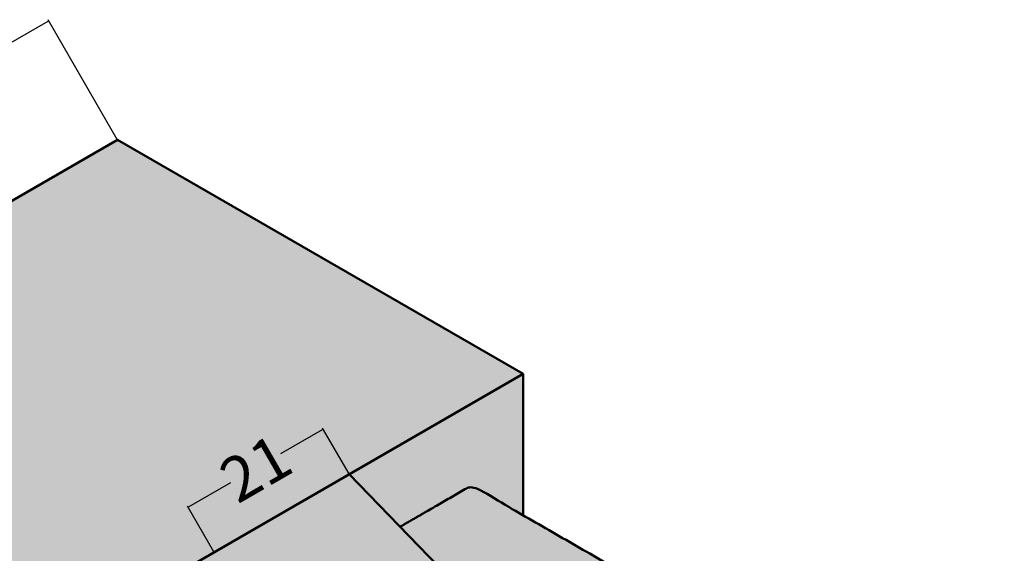
# Model space of a CAD drawing. Units: millimetres. Extents: x -24 to 183, y 0 to 191.
# Tile 1 of 1: x 51 to 183.4, y 119.6 to 191.4. Entities that reach past the tile are written whole.
import ezdxf

# ---------------------------------------------------------------- set-up
doc = ezdxf.new("R2010")
doc.units = ezdxf.units.MM
doc.header["$MEASUREMENT"] = 0
for name, color, linetype, lineweight in [('M-DIMS', 2, 'Continuous', 25), ('M-HATC', 7, 'Continuous', 18), ('M-OUTL', 7, 'Continuous', 50)]:
    doc.layers.add(name, color=color, linetype=linetype, lineweight=lineweight)
doc.styles.get("Standard").update_dxf_attribs({"font": 'arial.ttf'})
doc.dimstyles.get("Standard").update_dxf_attribs({"dimtxt": 6, "dimasz": 0.18, "dimexe": 0.18, "dimexo": 0.0625, "dimgap": 0.09, "dimtad": 0, "dimtoh": 1, "dimdec": 0, "dimzin": 0, "dimdsep": 46, "dimtxsty": 'Standard', "dimcen": 0.09, "dimadec": 0, "dimazin": 0, "dimtfac": 1, "dimtdec": 0, "dimtofl": 0, "dimtmove": 0, "dimatfit": 3, "dimfxl": 1, "dimtolj": 1, "dimtzin": 0, "dimarcsym": 0})

# ---------------------------------------------------------------- blocks, each defined once
blk = doc.blocks.new('*D1')
at = {"layer": 'Defpoints', "color": 0, "transparency": 16777216}
for p in [(91.82160620577477, 136.269941405224), (95.31936918098474, 130.2116382193271), (77.13283570151162, 119.7116382193271)]:
    blk.add_point(p, dxfattribs=at)
at = {"layer": 'M-DIMS', "color": 0, "lineweight": -2, "transparency": 16777216}
for p, q in [((91.66572163309357, 136.179941405224), (86.07071311753079, 132.9496617326455)), ((95.28811918098474, 130.2657648070636), (91.73160620577475, 136.4258259779052)), ((73.79095729898287, 125.859941405224), (79.38596581454564, 129.0902210778024)), ((77.10158570151162, 119.7657648070636), (73.54507272630167, 125.9258259779052))]:
    blk.add_line(p, q, dxfattribs=at)
at = {"layer": 'M-DIMS', "color": 0, "transparency": 16777216}
for points in [[(91.6507216330936, 136.2059221673375), (91.68072163309358, 136.1539606431104), (91.82160620577477, 136.269941405224)], [(73.77595729898287, 125.8859221673375), (73.80595729898288, 125.8339606431105), (73.63507272630167, 125.769941405224)]]:
    blk.add_solid(points, dxfattribs=at)
at = {"layer": 'M-DIMS', "color": 0, "transparency": 16777216, "insert": (82.72833946603824, 131.019941405224), "char_height": 6, "attachment_point": 5, "rotation": 30.00000000000005}
blk.add_mtext('\\A1;21', dxfattribs=at)
blk = doc.blocks.new('*D3')
at = {"layer": 'Defpoints', "color": 0, "transparency": 16777216}
for p in [(54.90112838051421, 191.2180848382955), (64.142454644745, 175.211638219327), (-0.8094506390879203, 137.7116382193271)]:
    blk.add_point(p, dxfattribs=at)
at = {"layer": 'M-DIMS', "color": 0, "lineweight": -2, "transparency": 16777216}
for p, q in [((54.745243807833, 191.1280848382955), (26.22301022659634, 174.6607656022791)), ((64.111204644745, 175.2657648070636), (54.8111283805142, 191.3739694109767)), ((-9.89489233063751, 153.8080848382955), (18.62734125059916, 170.2754040743118)), ((-0.8407006390879203, 137.7657648070636), (-10.14077690331872, 153.8739694109767))]:
    blk.add_line(p, q, dxfattribs=at)
at = {"layer": 'M-DIMS', "color": 0, "transparency": 16777216}
for points in [[(54.730243807833, 191.154065600409), (54.760243807833, 191.102104076182), (54.90112838051421, 191.2180848382955)], [(-9.909892330637511, 153.834065600409), (-9.87989233063751, 153.7821040761819), (-10.05077690331871, 153.7180848382955)]]:
    blk.add_solid(points, dxfattribs=at)
at = {"layer": 'M-DIMS', "color": 0, "transparency": 16777216, "insert": (22.42517573859776, 172.4680848382955), "char_height": 6, "attachment_point": 5, "rotation": 29.999999999999993}
blk.add_mtext('\\A1;75', dxfattribs=at)

msp = doc.modelspace()

# ---------------------------------------------------------------- hatches: boundary and pattern name
at = {"layer": 'M-HATC'}
h = msp.add_hatch(color=256, dxfattribs=at)
h.set_gradient(color1=(244, 238, 81), color2=(244, 238, 81), tint=1)
h.paths.add_polyline_path([(64.14245464474502, 175.211638219327), (-0.8094506390879131, 137.7116382193271), (53.75014979933173, 106.2116382193271), (118.7020550831646, 143.7116382193271)])
edge = h.paths.add_edge_path()
edge.add_line((95.31936918098478, 130.2116382193271), (77.13283570151161, 119.7116382193271))
edge.add_spline(control_points=[(77.13283570151158, 119.7116382193271), (89.17924906810929, 107.2566382193724), (101.2256624347508, 94.80163821937239)], knot_values=[5.356194490192345, 5.356194490192345, 5.356194490192345, 6.356194490188707, 6.356194490192345, 6.356194490192345], weights=[1, 1, 1], degree=2, periodic=0)
edge.add_spline(control_points=[(101.2256624347947, 94.80163821932707), (110.3189291745312, 100.051638219327), (119.4121959142679, 105.301638219327)], knot_values=[6.356194490188707, 6.356194490192345, 6.356194490192345, 7.356194490192345, 7.356194490192345, 7.356194490192345], weights=[1, 1, 1], degree=2, periodic=0)
edge.add_line((119.4121959142679, 105.3016382193271), (95.31936918098478, 130.2116382193271))
edge = h.paths.add_edge_path()
edge.add_spline(control_points=[(150.7449950231889, 106.2116382193271), (134.7235250531767, 115.4616382193271), (118.7020550831646, 124.7116382193271)], knot_values=[3.356194490192345, 3.356194490192345, 3.356194490192345, 4.178416712414569, 4.178416712414569, 4.178416712414569], weights=[1, 1, 1], degree=2, periodic=0)
edge.add_spline(control_points=[(118.7020550831646, 124.7116382193271), (115.2379534680269, 126.7116382193271), (111.7738518528891, 128.7116382193271)], knot_values=[4.178416712414569, 4.178416712414569, 4.178416712414569, 4.356194490192345, 4.356194490192345, 4.356194490192345], weights=[1, 1, 1], degree=2, periodic=0)
edge.add_spline(control_points=[(111.7738518528891, 128.7116382193271), (106.960071285434, 125.9324007128871), (102.1462907179789, 123.1531632064471)], knot_values=[4.356194490192345, 4.356194490192345, 4.356194490192345, 5.356194490192345, 5.356194490192345, 5.356194490192345], weights=[1, 1, 1], degree=2, periodic=0)
edge.add_line((102.1462907179789, 123.1531632064471), (119.4121959142679, 105.301638219327))
edge.add_spline(control_points=[(119.4121959142679, 105.301638219327), (126.8513541327762, 101.006638219327), (134.2905123512845, 96.71163821932709)], knot_values=[7.356194490192345, 7.356194490192345, 7.356194490192345, 8.356194490192346, 8.356194490192346, 8.356194490192346], weights=[1, 1, 1], degree=2, periodic=0)
edge.add_spline(control_points=[(134.2905123512845, 96.71163821932709), (158.0953395036126, 82.96791485491796), (161.6862132372617, 53.72180942535438), (165.2770869709107, 24.47570399579081), (142.5556009483879, 29.39608484008592)], knot_values=[8.356194490192346, 8.356194490192346, 8.356194490192346, 9.775566349411587, 9.775566349411587, 11.19493820863083, 11.19493820863083, 11.19493820863083], weights=[1, 0.7585665602715825, 1, 0.7585665602715825, 1], degree=2, periodic=0)
edge.add_spline(control_points=[(153.8864302935499, 30.77051272237281), (162.1136716295021, 35.52051272237281), (170.3409129654543, 40.2705127223728)], knot_values=[0, 0, 0, 1, 1, 1], weights=[1, 1, 1], degree=2, periodic=0)
edge.add_spline(control_points=[(170.3409129654543, 40.2705127223728), (183.4344867248955, 47.83009105704043), (176.3482956693094, 71.67543553482938), (169.2621046137232, 95.5207800126183), (150.7449950231889, 106.2116382193271)], knot_values=[1, 1, 1, 2.178097245096171, 2.178097245096171, 3.356194490192345, 3.356194490192345, 3.356194490192345], weights=[1, 0.831469612302545, 1, 0.831469612302545, 1], degree=2, periodic=0)
edge = h.paths.add_edge_path(flags=17)
edge.add_spline(control_points=[(134.2905123512845, 96.71163821932709), (126.8513541327762, 101.006638219327), (119.4121959142679, 105.301638219327)], knot_values=[7.356194490192345, 7.356194490192345, 7.356194490192345, 8.356194490192346, 8.356194490192346, 8.356194490192346], weights=[1, 1, 1], degree=2, periodic=0)
edge.add_line((119.4121959142679, 105.301638219327), (119.4121959142679, 84.07281383496964))
edge.add_spline(control_points=[(119.4121959142679, 84.07281383496964), (123.0724490086632, 81.4513939238958), (126.4903518736498, 77.88262675949477)], knot_values=[2.966768687208849, 2.966768687208849, 2.966768687208849, 3.231438789490306, 3.231438789490306, 3.231438789490306], weights=[0.9680864183363699, 0.938243390584542, 0.9254123758008628], degree=2, periodic=0)
edge.add_ellipse((134.2905123512845, 64.71163821932709), major_axis=(7.654655446197426, -13.25825214724777), ratio=0.5773502691896262, start_angle=359.3650130620468, end_angle=540.634986937953, ccw=False)
edge.add_spline(control_points=[(141.7968427812057, 51.37100682201758), (145.5119247027769, 38.61436904653682), (142.5556009483879, 29.39608484008592)], knot_values=[1.485548755374229, 1.485548755374229, 1.485548755374229, 2.169061485720957, 2.169061485720957, 2.169061485720957], weights=[0.9974346422091759, 0.9011559533067647, 0.9183363162707197], degree=2, periodic=0)
edge.add_spline(control_points=[(142.5556009483879, 29.39608484008592), (165.2770869709107, 24.47570399579081), (161.6862132372617, 53.72180942535438), (158.0953395036126, 82.96791485491796), (134.2905123512845, 96.71163821932709)], knot_values=[8.356194490192342, 8.356194490192342, 8.356194490192342, 9.775566349411587, 9.775566349411587, 11.19493820863083, 11.19493820863083, 11.19493820863083], weights=[1, 0.7585665602715825, 1, 0.7585665602715825, 1], degree=2, periodic=0)
edge = h.paths.add_edge_path()
edge.add_spline(control_points=[(119.4121959142679, 105.301638219327), (110.3189291745312, 100.051638219327), (101.2256624347947, 94.80163821932707)], knot_values=[6.356194490188707, 6.356194490188707, 6.356194490188707, 7.356194490188707, 7.356194490188707, 7.356194490192345], weights=[1, 1, 1], degree=2, periodic=0)
edge.add_spline(control_points=[(101.2256624347947, 94.80163821932709), (108.664820653303, 90.5066382193271), (116.1039788718113, 86.21163821932711)], knot_values=[3.356194490192346, 3.356194490192346, 3.356194490192346, 3.737972267970123, 3.737972267970123, 3.737972267970123], weights=[1, 1, 1], degree=2, periodic=0)
edge.add_spline(control_points=[(116.1039788718113, 86.21163821932711), (117.7640226821475, 85.25321147856292), (119.4121959142679, 84.07281383496964)], knot_values=[3.231438789490306, 3.231438789490306, 3.231438789490306, 3.356194490192346, 3.356194490192346, 3.356194490192346], weights=[1, 0.9821533182474542, 0.9680864183363699], degree=2, periodic=0)
edge.add_line((119.4121959142679, 84.07281383496965), (119.4121959142679, 105.301638219327))
h.paths.add_polyline_path([(-0.8094506390879131, 137.7116382193271), (-0.8094506390879131, 117.7116382193271), (32.09951470472076, 98.71163821932709), (32.09951470472076, 63.71163821932707), (-0.8094506390879131, 82.71163821932709), (-0.8094506390879062, 62.71163821932709), (53.75014979933173, 31.21163821932709), (53.75014979933173, 106.2116382193271)])
h.paths.add_polyline_path([(32.09951470472076, 98.71163821932709), (29.50143849336745, 100.2116382193271), (-0.8094506390879203, 82.71163821932709), (32.09951470472076, 63.71163821932708)])
edge = h.paths.add_edge_path()
edge.add_spline(control_points=[(99.64949619990696, 57.21163821932711), (99.64949619990696, 66.96163821932711), (99.64949619990696, 76.71163821932711)], knot_values=[5.141592653589794, 5.141592653589794, 5.141592653589794, 5.446280153589794, 5.446280153589794, 5.446280153589794], weights=[1, 1, 1], degree=2, periodic=0)
edge.add_line((99.64949619990699, 76.7116382193271), (60.67835302960723, 99.2116382193271))
edge.add_spline(control_points=[(60.67835302960723, 99.2116382193271), (60.67835302960723, 67.2116382193271), (60.67835302960723, 35.2116382193271)], knot_values=[0, 0, 0, 1, 1, 1], weights=[1, 1, 1], degree=2, periodic=0)
edge.add_spline(control_points=[(60.67835302960723, 35.2116382193271), (80.16392461475712, 23.9616382193271), (99.64949619990699, 12.71163821932711)], knot_values=[1, 1, 1, 2, 2, 2], weights=[1, 1, 1], degree=2, periodic=0)
edge.add_spline(control_points=[(99.64949619990699, 12.7116382193271), (99.64949619990699, 22.4616382193271), (99.64949619990699, 32.2116382193271)], knot_values=[5.836905153589794, 5.836905153589794, 5.836905153589794, 6.141592653589794, 6.141592653589794, 6.141592653589794], weights=[1, 1, 1], degree=2, periodic=0)
edge.add_ellipse((99.64949619990699, 44.7116382193271), major_axis=(7.654655446197426, -13.25825214724777), ratio=0.5773502691896261, start_angle=150, end_angle=330, ccw=False)
edge = h.paths.add_edge_path(flags=17)
edge.add_spline(control_points=[(77.13283570151158, 119.7116382193271), (77.13283570151158, 114.2116382193271), (77.13283570151158, 108.711638219327)], knot_values=[4.356194490192345, 4.356194490192345, 4.356194490192345, 5.356194490192345, 5.356194490192345, 5.356194490192345], weights=[1, 1, 1], degree=2, periodic=0)
edge.add_spline(control_points=[(77.13283570151158, 108.711638219327), (89.17924906815313, 101.7566382193271), (101.2256624347947, 94.80163821932709)], knot_values=[3.737972267970123, 3.737972267970123, 3.737972267970123, 4.356194490192345, 4.356194490192345, 4.356194490192345], weights=[1, 1, 1], degree=2, periodic=0)
edge.add_spline(control_points=[(101.2256624347508, 94.80163821937239), (89.17924906810929, 107.2566382193724), (77.13283570151158, 119.7116382193271)], knot_values=[5.356194490192345, 5.356194490192345, 5.356194490195983, 6.356194490192345, 6.356194490192345, 6.356194490192345], weights=[1, 1, 1], degree=2, periodic=0)
edge = h.paths.add_edge_path()
edge.add_spline(control_points=[(119.2454141421726, 10.77051272237291), (121.8252656817894, 12.25999070323999), (123.649496199907, 14.85523175877608), (131.649496199907, 26.23642960525908), (123.649496199907, 46.8552317587761), (115.649496199907, 67.4740339122931), (99.64949619990696, 76.71163821932711)], knot_values=[2.780860556892677, 2.780860556892677, 2.780860556892677, 3.047197551196599, 3.047197551196599, 4.094395102393195, 4.094395102393195, 5.141592653589794, 5.141592653589794, 5.141592653589794], weights=[0.9491840326991366, 0.9659258262890693, 1, 0.8660254037844385, 1, 0.8660254037844385, 1], degree=2, periodic=0)
edge.add_spline(control_points=[(99.64949619990696, 76.71163821932711), (99.64949619990696, 66.96163821932711), (99.64949619990696, 57.21163821932711)], knot_values=[5.141592653589794, 5.141592653589794, 5.141592653589794, 5.446280153589794, 5.446280153589794, 5.446280153589794], weights=[1, 1, 1], degree=2, periodic=0)
edge.add_ellipse((99.64949619990699, 44.7116382193271), major_axis=(7.654655446197426, -13.25825214724777), ratio=0.5773502691896261, start_angle=330, end_angle=509.9999999999999, ccw=False)
edge.add_spline(control_points=[(99.64949619990699, 32.2116382193271), (99.64949619990699, 22.4616382193271), (99.64949619990699, 12.7116382193271)], knot_values=[5.836905153589794, 5.836905153589794, 5.836905153589794, 6.141592653589794, 6.141592653589794, 6.141592653589794], weights=[1, 1, 1], degree=2, periodic=0)
edge.add_spline(control_points=[(99.64949619990699, 12.71163821932711), (111.1285191633359, 6.084221221357497), (119.2454141421726, 10.77051272237291)], knot_values=[2, 2, 2, 2.780860556892677, 2.780860556892677, 2.780860556892677], weights=[1, 0.9000995774953693, 0.9491840326991366], degree=2, periodic=0)
edge = h.paths.add_edge_path()
edge.add_line((118.7020550831646, 143.7116382193271), (95.31936918098478, 130.2116382193271))
edge.add_line((95.31936918098478, 130.2116382193271), (102.1462907179789, 123.1531632064471))
edge.add_spline(control_points=[(102.1462907179789, 123.1531632064471), (106.960071285434, 125.9324007128871), (111.7738518528891, 128.7116382193271)], knot_values=[4.356194490192345, 4.356194490192345, 4.356194490192345, 5.356194490192345, 5.356194490192345, 5.356194490192345], weights=[1, 1, 1], degree=2, periodic=0)
edge.add_spline(control_points=[(111.7738518528891, 128.7116382193271), (115.2379534680269, 126.7116382193271), (118.7020550831646, 124.7116382193271)], knot_values=[4.178416712414568, 4.178416712414568, 4.178416712414568, 4.356194490192344, 4.356194490192344, 4.356194490192344], weights=[1, 1, 1], degree=2, periodic=0)
edge.add_line((118.7020550831646, 124.7116382193271), (118.7020550831646, 143.7116382193271))
h = msp.add_hatch(color=256, dxfattribs=at)
h.set_gradient(color1=(244, 238, 81), color2=(244, 238, 81), tint=1)
edge = h.paths.add_edge_path()
edge.add_spline(control_points=[(77.13283570151158, 108.711638219327), (77.13283570151158, 114.2116382193271), (77.13283570151158, 119.7116382193271)], knot_values=[4.356194490192345, 4.356194490192345, 4.356194490192345, 5.356194490192345, 5.356194490192345, 5.356194490192345], weights=[1, 1, 1], degree=2, periodic=0)
edge.add_line((77.13283570151158, 119.7116382193271), (53.75014979933173, 106.2116382193271))
edge.add_line((53.75014979933173, 106.2116382193271), (53.75014979933173, 31.21163821932707))
edge.add_line((53.75014979933173, 31.21163821932707), (60.67835302960723, 35.21163821932709))
edge.add_spline(control_points=[(60.67835302960723, 35.2116382193271), (60.67835302960723, 67.2116382193271), (60.67835302960723, 99.2116382193271)], knot_values=[0, 0, 0, 1, 1, 1], weights=[1, 1, 1], degree=2, periodic=0)
edge.add_line((60.67835302960723, 99.2116382193271), (77.13283570151158, 108.7116382193271))
edge = h.paths.add_edge_path()
edge.add_spline(control_points=[(129.6626567046299, 74.29200746748931), (128.2121653973336, 76.06903189246286), (126.674769139423, 77.68917768712181)], knot_values=[2.842732393323176, 2.842732393323176, 2.842732393323176, 2.959718296587445, 2.959718296587445, 2.959718296587445], weights=[0.9171223116143046, 0.9192697655211874, 0.9247408519506481], degree=2, periodic=0)
edge.add_spline(control_points=[(126.674769139423, 77.68917768712181), (126.5826958679184, 77.78620675354577), (126.4903518736499, 77.88262675949478)], knot_values=[2.959718296587445, 2.959718296587445, 2.959718296587445, 2.966768687208849, 2.966768687208849, 2.966768687208849], weights=[0.9247408519506481, 0.925070577972116, 0.9254123758008624], degree=2, periodic=0)
edge.add_spline(control_points=[(126.4903518736499, 77.88262675949478), (125.1497541063207, 79.2823977540787), (123.7600353652503, 80.54602783327896)], knot_values=[2.966768687208849, 2.966768687208849, 2.966768687208849, 3.069712263544142, 3.069712263544142, 3.069712263544142], weights=[0.9254123758008624, 0.9304030057906388, 0.9379672558727182], degree=2, periodic=0)
edge.add_spline(control_points=[(123.7600353652503, 80.54602783327896), (122.2074968153256, 81.95770514094174), (120.6136211690738, 83.18146756875178)], knot_values=[3.069712263544142, 3.069712263544142, 3.069712263544142, 3.18671441540082, 3.18671441540082, 3.18671441540082], weights=[0.9379672558727182, 0.946564524087908, 0.9584863481523173], degree=2, periodic=0)
edge.add_spline(control_points=[(120.6136211690738, 83.18146756875178), (120.0147834077447, 83.6412494559974), (119.4121959142679, 84.07281383496966)], knot_values=[3.18671441540082, 3.18671441540082, 3.18671441540082, 3.231438789490306, 3.231438789490306, 3.231438789490306], weights=[0.9584863481523173, 0.9630434961263034, 0.9680864183363697], degree=2, periodic=0)
edge.add_spline(control_points=[(119.4121959142679, 84.07281383496966), (119.0199233503353, 84.35375372714144), (118.6264656481512, 84.62244284625048)], knot_values=[3.231438789490306, 3.231438789490306, 3.231438789490306, 3.260806039297188, 3.260806039297188, 3.260806039297188], weights=[0.9680864183363697, 0.9713977392729884, 0.9749185064116943], degree=2, periodic=0)
edge.add_spline(control_points=[(118.6264656481512, 84.62244284625048), (117.3678455130209, 85.48194447380494), (116.1039788718113, 86.21163821932711)], knot_values=[3.260806039297188, 3.260806039297188, 3.260806039297188, 3.356194490192345, 3.356194490192345, 3.356194490192345], weights=[0.9749185064116943, 0.9863543924933733, 1], degree=2, periodic=0)
edge.add_spline(control_points=[(116.1039788718113, 86.21163821932711), (111.8084928690405, 88.6916382193271), (107.5130068662697, 91.1716382193271)], knot_values=[3.356194490192345, 3.356194490192345, 3.356194490192345, 3.57663893463679, 3.57663893463679, 3.57663893463679], weights=[1, 1, 1], degree=2, periodic=0)
edge.add_spline(control_points=[(107.5130068662697, 91.1716382193271), (104.3693346505321, 92.98663821932709), (101.2256624347947, 94.80163821932709)], knot_values=[3.57663893463679, 3.57663893463679, 3.57663893463679, 3.737972267970123, 3.737972267970123, 3.737972267970123], weights=[1, 1, 1], degree=2, periodic=0)
edge.add_spline(control_points=[(101.2256624347947, 94.80163821932709), (89.18162767796578, 101.7552649283114), (77.13759292113684, 108.7088916372958)], knot_values=[3.737972267970123, 3.737972267970123, 3.737972267970123, 4.356072419879845, 4.356072419879845, 4.356072419879845], weights=[1, 1, 1], degree=2, periodic=0)
edge.add_line((77.13283570151157, 108.711638219327), (60.67835302960723, 99.2116382193271))
edge.add_line((60.67835302960723, 99.2116382193271), (99.8447195771881, 76.59892594990174))
edge.add_spline(control_points=[(99.97475492957814, 76.52164590242904), (100.1378798240307, 76.42525480692514), (100.3009708718766, 76.32666585249011)], knot_values=[5.117048971623415, 5.117048971623415, 5.117048971623415, 5.129320817599855, 5.129320817599855, 5.129320817599855], weights=[0.9968967702000623, 0.9953635526324084, 0.9938671322846566], degree=2, periodic=0)
edge.add_spline(control_points=[(100.3009708718766, 76.32666585249011), (100.6286285674363, 76.12859593973583), (100.9560124019527, 75.92173877705902)], knot_values=[5.092505444169316, 5.092505444169316, 5.092505444169316, 5.117048971623414, 5.117048971623414, 5.117048971623414], weights=[0.9938671322846566, 0.9908743116480199, 0.988028677917995], degree=2, periodic=0)
edge.add_spline(control_points=[(100.9560124019527, 75.92173877705902), (101.2862460391653, 75.71308096927459), (101.6160138777021, 75.49560053592234)], knot_values=[5.067890674546034, 5.067890674546034, 5.067890674546034, 5.092505444169316, 5.092505444169316, 5.092505444169316], weights=[0.988028677917995, 0.9851747842049658, 0.9824689331136189], degree=2, periodic=0)
edge.add_spline(control_points=[(101.6160138777021, 75.49560053592234), (102.1164304547191, 75.16557801307957), (102.6152306653907, 74.81560168592624)], knot_values=[5.030795417572638, 5.030795417572638, 5.030795417572638, 5.067890674546034, 5.067890674546034, 5.067890674546034], weights=[0.9824689331136189, 0.9783911276699186, 0.9746495487607924], degree=2, periodic=0)
edge.add_spline(control_points=[(102.6152306653907, 74.81560168592624), (103.6180936700229, 74.11195661222713), (104.6104560145192, 73.33052013900783)], knot_values=[4.957065639950063, 4.957065639950063, 4.957065639950063, 5.030795417572638, 5.030795417572638, 5.030795417572638], weights=[0.9746495487607924, 0.9672128626872858, 0.9611044304061584], degree=2, periodic=0)
edge.add_spline(control_points=[(104.6104560145192, 73.33052013900783), (105.6134251683119, 72.5407313258447), (106.6002754642349, 71.67572813658762)], knot_values=[4.883488068876007, 4.883488068876007, 4.883488068876007, 4.957065639950062, 4.957065639950062, 4.957065639950062], weights=[0.9611044304061584, 0.9550086082728485, 0.9502355615416473], degree=2, periodic=0)
edge.add_spline(control_points=[(106.6002754642349, 71.67572813658762), (108.106571986875, 70.35541511501445), (109.5597114832291, 68.87391790201954)], knot_values=[4.772588940897321, 4.772588940897321, 4.772588940897321, 4.883488068876008, 4.883488068876008, 4.883488068876008], weights=[0.9502355615416473, 0.9430414300615662, 0.9388523470348884], degree=2, periodic=0)
edge.add_spline(control_points=[(109.5597114832291, 68.87391790201954), (110.8516035735683, 67.55681480480848), (112.0878073272173, 66.12614290817397)], knot_values=[4.674819786984862, 4.674819786984862, 4.674819786984862, 4.772588940897322, 4.772588940897322, 4.772588940897322], weights=[0.9388523470348884, 0.9351592332056611, 0.9338017218698066], degree=2, periodic=0)
edge.add_spline(control_points=[(112.0878073272173, 66.12614290817397), (113.638943035053, 64.33099687458838), (115.0807423105997, 62.38251306400263)], knot_values=[4.55254402668912, 4.55254402668912, 4.55254402668912, 4.674819786984861, 4.674819786984861, 4.674819786984861], weights=[0.9338017218698066, 0.932103939654668, 0.9340593785643667], degree=2, periodic=0)
edge.add_spline(control_points=[(115.0807423105997, 62.38251306400263), (116.5292798236757, 60.42492302971401), (117.8446599635839, 58.34337763107811)], knot_values=[4.42917907937402, 4.42917907937402, 4.42917907937402, 4.55254402668912, 4.55254402668912, 4.55254402668912], weights=[0.9340593785643667, 0.9360322357969812, 0.9417236870938861], degree=2, periodic=0)
edge.add_spline(control_points=[(117.8446599635839, 58.34337763107811), (118.8713225058487, 56.71871824481724), (119.8054692643808, 55.03626807420435)], knot_values=[4.331844561881248, 4.331844561881248, 4.331844561881248, 4.42917907937402, 4.42917907937402, 4.42917907937402], weights=[0.9417236870938861, 0.9462142225164228, 0.9530196405744161], degree=2, periodic=0)
edge.add_spline(control_points=[(119.8054692643808, 55.03626807420435), (121.1922080878205, 52.53867446936446), (122.3511098193492, 49.95830163102931)], knot_values=[4.184741853008914, 4.184741853008914, 4.184741853008914, 4.331844561881248, 4.331844561881248, 4.331844561881248], weights=[0.9530196405744161, 0.9633047424799539, 0.9788771760901379], degree=2, periodic=0)
edge.add_spline(control_points=[(122.3511098193492, 49.95830163102931), (123.0447771856724, 48.41380447289763), (123.649496199907, 46.8552317587761), (123.7106124829862, 46.69771369013003), (123.7707926063305, 46.54011834809961)], knot_values=[4.085168284068898, 4.085168284068898, 4.085168284068898, 4.175515034684617, 4.175515034684617, 4.184741853008914, 4.184741853008914, 4.184741853008914], weights=[0.9788771760901379, 0.9884413696161741, 1, 0.9988195548605517, 0.9976599114367514], degree=2, periodic=0)
edge.add_spline(control_points=[(123.7707926063305, 46.54011834809961), (124.5776705294812, 44.42712496740803), (125.2107977955467, 42.31611465871429)], knot_values=[3.9634953926215, 3.9634953926215, 3.9634953926215, 4.085168284068899, 4.085168284068899, 4.085168284068899], weights=[0.9976599114367514, 0.9823678396236314, 0.9706930540319149], degree=2, periodic=0)
edge.add_spline(control_points=[(125.2107977955467, 42.31611465871429), (125.6736053367575, 40.77299443186174), (126.0393314773653, 39.24456708280777)], knot_values=[3.876368048263354, 3.876368048263354, 3.876368048263354, 3.9634953926215, 3.9634953926215, 3.9634953926215], weights=[0.9706930540319149, 0.9623329908127651, 0.9558277578449111], degree=2, periodic=0)
edge.add_spline(control_points=[(126.0393314773653, 39.24456708280777), (126.3548486882267, 37.92597078729458), (126.5961836872144, 36.62622374004979)], knot_values=[3.80214301191095, 3.80214301191095, 3.80214301191095, 3.876368048263354, 3.876368048263354, 3.876368048263354], weights=[0.9558277578449111, 0.9502858564237563, 0.9460901130582945], degree=2, periodic=0)
edge.add_spline(control_points=[(126.5961836872144, 36.62622374004979), (126.9174285486043, 34.89610974172617), (127.1046069641274, 33.21425510536911)], knot_values=[3.70435185738841, 3.70435185738841, 3.70435185738841, 3.802143011910949, 3.802143011910949, 3.802143011910949], weights=[0.9460901130582945, 0.9405622398775964, 0.9373710204515152], degree=2, periodic=0)
edge.add_spline(control_points=[(127.1046069641274, 33.21425510536911), (127.2465779563155, 31.9386028311868), (127.3104091259611, 30.69911679832556)], knot_values=[3.630620672153618, 3.630620672153618, 3.630620672153618, 3.70435185738841, 3.70435185738841, 3.70435185738841], weights=[0.9373710204515152, 0.9349649501706391, 0.9338871843993468], degree=2, periodic=0)
edge.add_spline(control_points=[(127.3104091259611, 30.69911679832556), (127.3955283033867, 29.04625610137234), (127.3411002741898, 27.47218361842691)], knot_values=[3.532563843898478, 3.532563843898478, 3.532563843898478, 3.630620672153617, 3.630620672153617, 3.630620672153617], weights=[0.9338871843993468, 0.9324538384847469, 0.9333698597606337], degree=2, periodic=0)
edge.add_spline(control_points=[(127.3411002741898, 27.47218361842691), (127.300188233985, 26.28899698356999), (127.180615341149, 25.15821918772291)], knot_values=[3.458730317071423, 3.458730317071423, 3.458730317071423, 3.532563843898478, 3.532563843898478, 3.532563843898478], weights=[0.9333698597606337, 0.9340595932820093, 0.9360813213430013], degree=2, periodic=0)
edge.add_spline(control_points=[(127.180615341149, 25.15821918772291), (127.044748511288, 23.87335277063611), (126.8083021586305, 22.66499248616322)], knot_values=[3.374446783935056, 3.374446783935056, 3.374446783935056, 3.458730317071423, 3.458730317071423, 3.458730317071423], weights=[0.9360813213430013, 0.9383891940851565, 0.9424327908815358], degree=2, periodic=0)
edge.add_spline(control_points=[(126.8083021586305, 22.66499248616322), (126.6325923480817, 21.76702660818197), (126.4021292816593, 20.91561921939569)], knot_values=[3.311341395677428, 3.311341395677428, 3.311341395677428, 3.374446783935056, 3.374446783935056, 3.374446783935056], weights=[0.9424327908815358, 0.9454603424838158, 0.9494609282808749], degree=2, periodic=0)
edge.add_spline(control_points=[(126.4021292816593, 20.91561921939569), (126.2248036377586, 20.26051918197064), (126.0155393341565, 19.63480491824097)], knot_values=[3.262421368203812, 3.262421368203812, 3.262421368203812, 3.311341395677428, 3.311341395677428, 3.311341395677428], weights=[0.9494609282808749, 0.9525622287007962, 0.9562482769267935], degree=2, periodic=0)
edge.add_spline(control_points=[(126.0155393341565, 19.63480491824097), (125.7802944825154, 18.93140707825095), (125.5053695818401, 18.26715694529732)], knot_values=[3.206973826924972, 3.206973826924972, 3.206973826924972, 3.262421368203813, 3.262421368203813, 3.262421368203813], weights=[0.9562482769267935, 0.9604261631979532, 0.9653552567738074], degree=2, periodic=0)
edge.add_spline(control_points=[(125.5053695818401, 18.26715694529732), (125.2647817315435, 17.68586906939387), (124.9944008162674, 17.13601478791239)], knot_values=[3.157982411241067, 3.157982411241067, 3.157982411241067, 3.206973826924972, 3.206973826924972, 3.206973826924972], weights=[0.9653552567738074, 0.9697104232383605, 0.9746520453803764], degree=2, periodic=0)
edge.add_spline(control_points=[(124.9944008162674, 17.13601478791239), (124.7917726002789, 16.72394431320289), (124.5727165965067, 16.33016080220038)], knot_values=[3.120938813188745, 3.120938813188745, 3.120938813188745, 3.157982411241067, 3.157982411241067, 3.157982411241067], weights=[0.9746520453803764, 0.9783885257780115, 0.9824602969029337], degree=2, periodic=0)
edge.add_spline(control_points=[(124.5727165965067, 16.33016080220038), (124.3091183628697, 15.85630646290719), (124.0221924242566, 15.40974891923198)], knot_values=[3.075952071171273, 3.075952071171273, 3.075952071171273, 3.120938813188746, 3.120938813188746, 3.120938813188746], weights=[0.9824602969029337, 0.987405165295371, 0.9928445314164283], degree=2, periodic=0)
edge.add_spline(control_points=[(124.0221924242566, 15.40974891923198), (123.8404369956832, 15.12687363048792), (123.649496199907, 14.85523175877608), (123.5683140978384, 14.73973806312165), (123.4854899919731, 14.62630190952734)], knot_values=[3.034946113864857, 3.034946113864857, 3.034946113864857, 3.063700633839531, 3.063700633839531, 3.075952071171272, 3.075952071171272, 3.075952071171272], weights=[0.9928445314164283, 0.9963212526628074, 1, 0.998432596249194, 0.9969018674291203], degree=2, periodic=0)
edge.add_spline(control_points=[(123.4854899919731, 14.62630190952734), (123.2328877991915, 14.28033715881531), (122.9652307127422, 13.95379879127234)], knot_values=[2.997811825835947, 2.997811825835947, 2.997811825835947, 3.034946113864858, 3.034946113864858, 3.034946113864858], weights=[0.9969018674291203, 0.992262205701308, 0.9879594784250201], degree=2, periodic=0)
edge.add_spline(control_points=[(122.9652307127422, 13.95379879127234), (122.6092507510389, 13.51950759758628), (122.2273513432456, 13.1204294435816)], knot_values=[2.948919902028313, 2.948919902028313, 2.948919902028313, 2.997811825835947, 2.997811825835947, 2.997811825835947], weights=[0.9879594784250201, 0.9822944010713484, 0.9772133998627793], degree=2, periodic=0)
edge.add_spline(control_points=[(122.2273513432456, 13.1204294435816), (121.9363818855874, 12.81637148574149), (121.6308038631775, 12.53322017569058)], knot_values=[2.912007262502068, 2.912007262502068, 2.912007262502068, 2.948919902028313, 2.948919902028313, 2.948919902028313], weights=[0.9772133998627793, 0.9733773232382992, 0.9698741708558454], degree=2, periodic=0)
edge.add_spline(control_points=[(121.6308038631775, 12.53322017569058), (121.2205195242283, 12.15304706261559), (120.7847527856912, 11.81133624302551)], knot_values=[2.862862349391971, 2.862862349391971, 2.862862349391971, 2.912007262502068, 2.912007262502068, 2.912007262502068], weights=[0.9698741708558454, 0.9652101283582961, 0.9611362222017703], degree=2, periodic=0)
edge.add_spline(control_points=[(120.7847527856912, 11.81133624302551), (120.4564077324761, 11.55386120576316), (120.1141041105082, 11.31863046503682)], knot_values=[2.826105434023206, 2.826105434023206, 2.826105434023206, 2.862862349391971, 2.862862349391971, 2.862862349391971], weights=[0.9611362222017703, 0.9580892288439788, 0.9553723566239481], degree=2, periodic=0)
edge.add_spline(control_points=[(120.1141041105082, 11.31863046503682), (119.7699713416554, 11.08214273621856), (119.4121959142679, 10.86845743728019)], knot_values=[2.789361644115605, 2.789361644115605, 2.789361644115605, 2.826105434023205, 2.826105434023205, 2.826105434023205], weights=[0.9553723566239481, 0.9526564545669589, 0.9502704379250916], degree=2, periodic=0)
edge.add_spline(control_points=[(119.4121959142679, 10.86680422338807), (123.4424256961962, 13.19365847288044), (127.4726554781246, 15.52051272237282)], knot_values=[0.0101359474752899, 0.0101359474752899, 0.0101359474752899, 0.5, 0.5, 0.5], weights=[1, 1, 1], degree=2, periodic=0)
edge.add_spline(control_points=[(127.4726554781246, 15.52051272237282), (131.5862761461006, 17.89551272237281), (135.6998968140767, 20.27051272237281)], knot_values=[0.5, 0.5, 0.5, 1, 1, 1], weights=[1, 1, 1], degree=2, periodic=0)
edge.add_spline(control_points=[(135.6998968140767, 20.27051272237281), (136.1539621123821, 20.53266744457909), (136.5865086976751, 20.83096823723133)], knot_values=[1, 1, 1, 1.048792481471118, 1.048792481471118, 1.048792481471118], weights=[1, 0.9930200873881364, 0.9866183397082462], degree=2, periodic=0)
edge.add_spline(control_points=[(136.5865086976751, 20.83096823723133), (136.9176670820245, 21.05934781969398), (137.2357290184705, 21.30858758031019)], knot_values=[1.048792481471118, 1.048792481471118, 1.048792481471118, 1.085724978803377, 1.085724978803377, 1.085724978803377], weights=[0.9866183397082462, 0.9817726642684901, 0.9772582444714648], degree=2, periodic=0)
edge.add_spline(control_points=[(137.2357290184705, 21.30858758031019), (137.7660086555937, 21.72412541955322), (138.2584225013502, 22.19645227598328)], knot_values=[1.085724978803377, 1.085724978803377, 1.085724978803377, 1.146550188018983, 1.146550188018983, 1.146550188018983], weights=[0.9772582444714648, 0.9698233145729854, 0.9632868744875692], degree=2, periodic=0)
edge.add_spline(control_points=[(138.2584225013502, 22.19645227598328), (138.5573675401466, 22.4832024793678), (138.8418384740707, 22.79040575169065)], knot_values=[1.146550188018983, 1.146550188018983, 1.146550188018983, 1.183078897280162, 1.183078897280162, 1.183078897280162], weights=[0.9632868744875692, 0.9593614014384435, 0.9557599803012227], degree=2, periodic=0)
edge.add_spline(control_points=[(138.8418384740707, 22.79040575169065), (139.1385886179396, 23.11086947710986), (139.4191808804897, 23.4531491801297)], knot_values=[1.183078897280162, 1.183078897280162, 1.183078897280162, 1.220893242354295, 1.220893242354295, 1.220893242354295], weights=[0.9557599803012227, 0.9520318063691403, 0.9486508959071877], degree=2, periodic=0)
edge.add_spline(control_points=[(139.4191808804897, 23.4531491801297), (139.8668572680979, 23.99924599551215), (140.2721260020161, 24.59926038119931)], knot_values=[1.220893242354295, 1.220893242354295, 1.220893242354295, 1.280671920731201, 1.280671920731201, 1.280671920731201], weights=[0.9486508959071877, 0.9433061951400592, 0.9388293321538448], degree=2, periodic=0)
edge.add_spline(control_points=[(140.2721260020161, 24.59926038119931), (140.5232608792327, 24.97107425793451), (140.7576523147468, 25.36293735961763)], knot_values=[1.280671920731201, 1.280671920731201, 1.280671920731201, 1.317431357422621, 1.317431357422621, 1.317431357422621], weights=[0.9388293321538448, 0.9360763947188564, 0.93365161576264], degree=2, periodic=0)
edge.add_spline(control_points=[(140.7576523147468, 25.36293735961763), (141.0830933170729, 25.90702004039749), (141.3755268808085, 26.48850448529568)], knot_values=[1.317431357422621, 1.317431357422621, 1.317431357422621, 1.368155388312501, 1.368155388312501, 1.368155388312501], weights=[0.93365161576264, 0.930305684112252, 0.9275845991199414], degree=2, periodic=0)
edge.add_spline(control_points=[(141.3755268808085, 26.48850448529568), (141.6466700533705, 27.02765442133951), (141.8887940808721, 27.59768818100019)], knot_values=[1.368155388312501, 1.368155388312501, 1.368155388312501, 1.414922102988684, 1.414922102988684, 1.414922102988684], weights=[0.9275845991199414, 0.9250758039155279, 0.9230981617358409], degree=2, periodic=0)
edge.add_spline(control_points=[(141.8887940808721, 27.59768818100019), (142.1766643775072, 28.2754226015726), (142.4226727061001, 28.99479987589269)], knot_values=[1.414922102988684, 1.414922102988684, 1.414922102988684, 1.470265260532734, 1.470265260532734, 1.470265260532734], weights=[0.9230981617358409, 0.9207578441943155, 0.9191613568443742], degree=2, periodic=0)
edge.add_spline(control_points=[(142.4226727061001, 28.99479987589269), (142.490760707178, 29.19390273110689), (142.5556009483879, 29.39608484008591)], knot_values=[1.470265260532734, 1.470265260532734, 1.470265260532734, 1.485548755374229, 1.485548755374229, 1.485548755374229], weights=[0.9191613568443742, 0.9187204729617025, 0.9183363162707195], degree=2, periodic=0)
edge.add_spline(control_points=[(142.5556009483879, 29.39608484008591), (142.7432960737653, 29.98134787405721), (142.9035286953098, 30.5915899432056)], knot_values=[1.485548755374229, 1.485548755374229, 1.485548755374229, 1.529718415129709, 1.529718415129709, 1.529718415129709], weights=[0.9183363162707195, 0.9172260943934935, 0.9165896714100165], degree=2, periodic=0)
edge.add_spline(control_points=[(142.9035286953098, 30.5915899432056), (143.3840015652817, 32.42145926391575), (143.6126416122373, 34.45248245982711)], knot_values=[1.529718415129709, 1.529718415129709, 1.529718415129709, 1.66179866791104, 1.66179866791104, 1.66179866791104], weights=[0.9165896714100165, 0.9146865798082515, 0.9170201297212321], degree=2, periodic=0)
edge.add_spline(control_points=[(143.6126416122373, 34.45248245982711), (143.713072375763, 35.34461493189241), (143.764143780702, 36.27047774601957)], knot_values=[1.66179866791104, 1.66179866791104, 1.66179866791104, 1.720028544551231, 1.720028544551231, 1.720028544551231], weights=[0.9170201297212321, 0.9180489157865613, 0.9199011526878917], degree=2, periodic=0)
edge.add_spline(control_points=[(143.764143780702, 36.27047774601957), (143.8286054170071, 37.43908926285298), (143.8141447210366, 38.65544637076558)], knot_values=[1.720028544551231, 1.720028544551231, 1.720028544551231, 1.793861813952505, 1.793861813952505, 1.793861813952505], weights=[0.9199011526878917, 0.9222497186478706, 0.9259221692199169], degree=2, periodic=0)
edge.add_spline(control_points=[(143.8141447210366, 38.65544637076558), (143.8028189982979, 39.60810614478695), (143.7430996364778, 40.58628027454679)], knot_values=[1.793861813952505, 1.793861813952505, 1.793861813952505, 1.852100472733457, 1.852100472733457, 1.852100472733457], weights=[0.9259221692199169, 0.9288189472915059, 0.932539424601013], degree=2, periodic=0)
edge.add_spline(control_points=[(143.7430996364778, 40.58628027454679), (143.6681967845851, 41.81315259423612), (143.517572054451, 43.07408489058984)], knot_values=[1.852100472733457, 1.852100472733457, 1.852100472733457, 1.925809061489029, 1.925809061489029, 1.925809061489029], weights=[0.932539424601013, 0.9372481719815517, 0.9432763365187515], degree=2, periodic=0)
edge.add_spline(control_points=[(143.517572054451, 43.07408489058984), (143.3419048088425, 44.54465684249924), (143.0645134371127, 46.05133158854439)], knot_values=[1.925809061489029, 1.925809061489029, 1.925809061489029, 2.012979034199378, 2.012979034199378, 2.012979034199378], weights=[0.9432763365187515, 0.9504054234687641, 0.9593798646914953], degree=2, periodic=0)
edge.add_spline(control_points=[(143.0645134371127, 46.05133158854439), (142.8323158915082, 47.31253223755684), (142.5301351100322, 48.59179692702449)], knot_values=[2.012979034199378, 2.012979034199378, 2.012979034199378, 2.08722275193102, 2.08722275193102, 2.08722275193102], weights=[0.9593798646914953, 0.9670235045851738, 0.9760057892826022], degree=2, periodic=0)
edge.add_spline(control_points=[(142.5301351100322, 48.59179692702449), (142.2034215698478, 49.97491961764523), (141.7968427812057, 51.37100682201758)], knot_values=[2.08722275193102, 2.08722275193102, 2.08722275193102, 2.169061485720957, 2.169061485720957, 2.169061485720957], weights=[0.9760057892826022, 0.9859069476383204, 0.9974346422091759], degree=2, periodic=0)
edge.add_spline(control_points=[(141.7968427812057, 51.37100682201758), (141.7525280489804, 51.52317223829919), (141.7072795179318, 51.67543553482938), (141.6624929613182, 51.82614426707313), (141.6167947871972, 51.97693808478169)], knot_values=[2.169061485720957, 2.169061485720957, 2.169061485720957, 2.178097245096171, 2.178097245096171, 2.187040870006556, 2.187040870006556, 2.187040870006556], weights=[0.9974346422091759, 0.9987074071881719, 1, 0.9987205873030927, 0.9974606001456546], degree=2, periodic=0)
edge.add_spline(control_points=[(141.6167947871972, 51.97693808478169), (140.9517794604651, 54.17134085647821), (140.0997815197228, 56.36604687055694)], knot_values=[2.187040870006556, 2.187040870006556, 2.187040870006556, 2.314683904073241, 2.314683904073241, 2.314683904073241], weights=[0.9974606001456546, 0.9794781170616754, 0.965452398201826], degree=2, periodic=0)
edge.add_spline(control_points=[(140.0997815197228, 56.36604687055694), (139.2839372106333, 58.46762285576458), (138.3081005691592, 60.53982325286182)], knot_values=[2.314683904073241, 2.314683904073241, 2.314683904073241, 2.433530685609216, 2.433530685609216, 2.433530685609216], weights=[0.965452398201826, 0.9523932324008108, 0.9427642772030161], degree=2, periodic=0)
edge.add_spline(control_points=[(138.3081005691592, 60.53982325286182), (137.0861762910274, 63.13459359325666), (135.6376199164575, 65.63298565436963)], knot_values=[2.433530685609216, 2.433530685609216, 2.433530685609216, 2.579002148155839, 2.579002148155839, 2.579002148155839], weights=[0.9427642772030161, 0.9309781928234816, 0.9243313797502773], degree=2, periodic=0)
edge.add_spline(control_points=[(135.6376199164575, 65.63298565436963), (134.4574971723731, 67.66839783902462), (133.1455600512967, 69.60716400973533)], knot_values=[2.579002148155839, 2.579002148155839, 2.579002148155839, 2.695989522507838, 2.695989522507838, 2.695989522507838], weights=[0.9243313797502773, 0.9189860481255712, 0.9169644326127578], degree=2, periodic=0)
edge.add_spline(control_points=[(133.1455600512967, 69.60716400973533), (131.4917327990659, 72.05117163579708), (129.6626567046299, 74.29200746748931)], knot_values=[2.695989522507838, 2.695989522507838, 2.695989522507838, 2.842732393323176, 2.842732393323176, 2.842732393323176], weights=[0.9169644326127578, 0.9144286233796822, 0.9171223116143046], degree=2, periodic=0)
h.paths.add_polyline_path([(76.47887617717802, 91.77949279967994), (87.15119196487902, 85.61782840677407), (93.33332020498817, 96.32558861754949), (82.66100441728715, 102.4872530104553)], flags=24)

# ---------------------------------------------------------------- linework, layer by layer
at = {"layer": 'M-OUTL'}
for points in [[(53.75014979933173, 106.2116382193271), (-0.8094506390879131, 137.7116382193271), (64.14245464474502, 175.211638219327), (118.7020550831646, 143.7116382193271), (118.7020550831646, 124.7116382193271)], [(60.67835302960723, 35.21163821932709), (53.75014979933173, 31.2116382193271), (53.75014979933173, 106.2116382193271), (118.7020550831646, 143.7116382193271)], [(95.31936918098476, 130.2116382193271), (119.4121959142679, 105.301638219327), (119.4121959142679, 84.07281383496965)]]:
    msp.add_lwpolyline(points, dxfattribs=at)
msp.add_rational_spline([(153.8864302935499, 30.77051272237281), (162.1136716295021, 35.52051272237281), (170.3409129654543, 40.2705127223728), (183.4344867248955, 47.83009105704043), (176.3482956693094, 71.67543553482938), (169.2621046137232, 95.5207800126183), (150.7449950231889, 106.2116382193271), (131.259423438039, 117.4616382193271), (111.7738518528891, 128.7116382193271), (106.960071285434, 125.9324007128871), (102.1462907179789, 123.1531632064471)], [1, 1, 1, 0.831469612302545, 1, 0.831469612302545, 1, 1, 1, 1, 1], degree=2, knots=[0, 0, 0, 1, 1, 2.178097245096171, 2.178097245096171, 3.356194490192345, 3.356194490192345, 4.356194490192345, 4.356194490192345, 5.356194490192345, 5.356194490192345, 5.356194490192345], dxfattribs=at)

# ---------------------------------------------------------------- dimensions: what is measured, and where the dimension line sits
at = {"layer": 'M-DIMS'}
for p1, p2, distance, picture, middle in [((-0.8094506390879131, 137.7116382193271), (64.14245464474502, 175.211638219327), 18.48265252846167, '*D3', (22.42517573859776, 172.4680848382955)), ((77.13283570151162, 119.7116382193271), (95.31936918098475, 130.2116382193271), 6.995525950419884, '*D1', (82.72833946603824, 131.019941405224))]:
    dim = msp.add_aligned_dim(p1=p1, p2=p2, distance=distance, dimstyle='Standard', override={"dimclrd": 0, "dimclre": 0, "dimclrt": 0}, dxfattribs=at)
    dim.commit()
    dim.dimension.update_dxf_attribs({"geometry": picture, "text_midpoint": middle})

doc.saveas('drawing.dxf')
